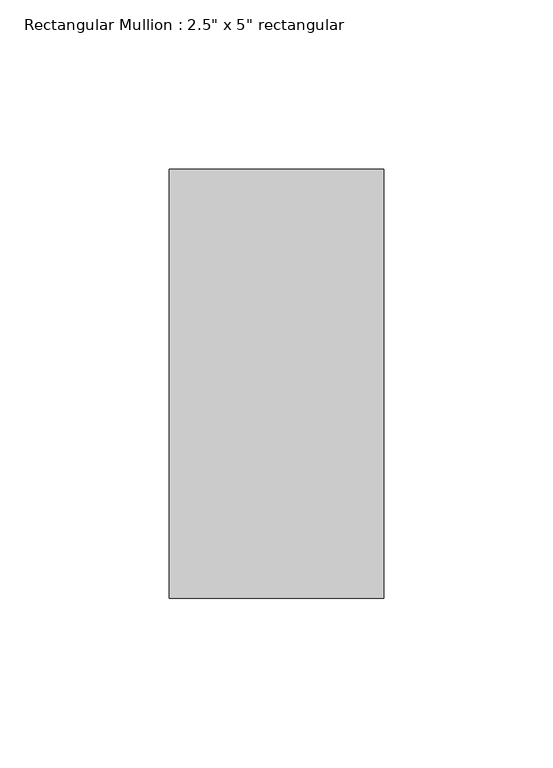
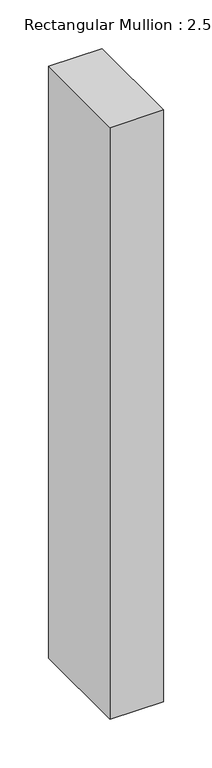
"""IFC4 building model written with IfcOpenShell, lengths in millimetres: member geometry."""

from ifc_helpers import new_model, si_unit, frame, origin, place, context, project, spatial, polyline, outline, extrude, source, transform, mapped, element, save


def member_7b995701(model_context):
    return source(origin(), model_context, "Body", "SweptSolid", [
        extrude(outline(polyline([(31.75, 63.5), (31.75, -63.5), (-31.75, -63.5), (-31.75, 63.5), (31.75, 63.5)])), frame((0.0, 0.0, -742.95), z_axis=(0.0, 0.0, 1.0), x_axis=(1.0, 0.0, 0.0)), (0.0, 0.0, 1.0), 742.95),
    ])


if __name__ == "__main__":
    model = new_model("IFC4")
    model_context = context("Model", 3, world=origin())
    ifc_project = project(units=[si_unit("LENGTHUNIT", "METRE", prefix="MILLI")], contexts=[model_context])
    site = spatial("IfcSite", under=ifc_project)
    building = spatial("IfcBuilding", under=site)
    placement = place(None, origin())
    member_shape = member_7b995701(model_context)
    element("IfcMember", 1, ObjectType="Rectangular Mullion : 2.5\" x 5\" rectangular", at=placement, inside=building, context=model_context, shape_type="MappedRepresentation", body=[
        mapped(member_shape, transform((0.0, 0.0, 0.0), x_axis=(1.0, 0.0, 0.0), y_axis=(0.0, 1.0, 0.0), z_axis=(0.0, 0.0, 1.0))),
    ])
    save(model, "model.ifc")

# Revit data of these elements
# Type "Rectangular Mullion : 2.5\" x 5\" rectangular"
#   built-in parameter 1007304 = 0.416667 (stored number, unit not read)
#   built-in parameter 1007301 = 0.104167 (stored number, unit not read)
#   built-in parameter 1007300 = 0.104167 (stored number, unit not read)
# Element 1 (IfcMember, "Rectangular Mullion : 2.5\" x 5\" rectangular")
#   Materials on its faces: "Aluminum"
# Materials
#   "Aluminum": class "Metal", colour RGB 247 247 247, transparency 0, Description = "Aluminum 6061", Cost = 0
